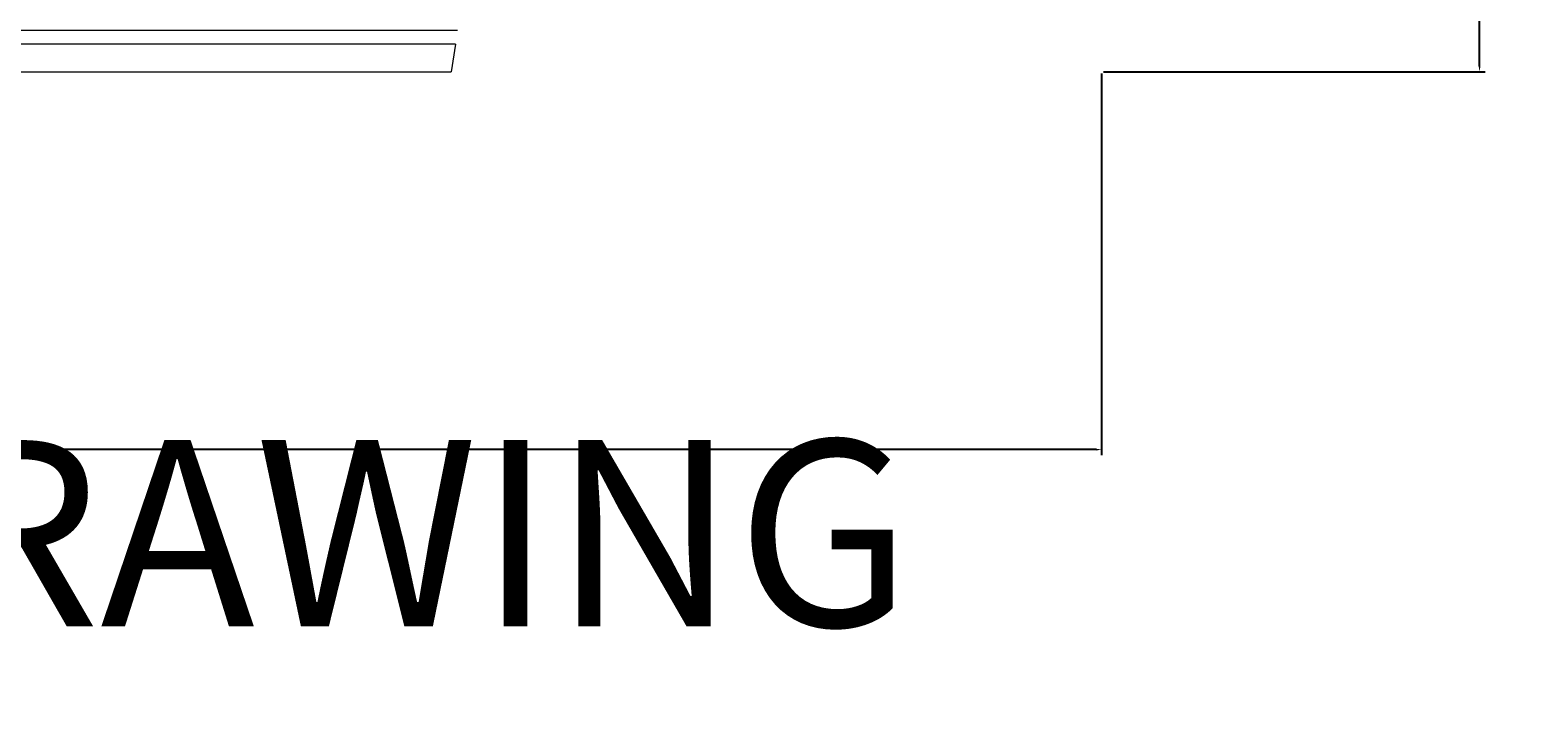
# Model space of a CAD drawing. Units: inches. Extents: x 4159 to 4826, y 299 to 1026.
# Tile 22 of 37: x 4354 to 4402, y 559 to 581. Entities that reach past the tile are written whole.
import ezdxf

# ---------------------------------------------------------------- set-up
doc = ezdxf.new("R2010")
doc.units = ezdxf.units.IN
for name, color, linetype, lineweight in [('A-ANNO-DIMS', 2, 'Continuous', 18), ('A-AREA-IDEN', 7, 'Continuous', 18), ('A-FURN', 8, 'Continuous', 18)]:
    doc.layers.add(name, color=color, linetype=linetype, lineweight=lineweight)
doc.styles.get("Standard").update_dxf_attribs({"font": 'arial.ttf'})
doc.dimstyles.get("Standard").update_dxf_attribs({"dimtxt": 0.18, "dimasz": 0.18, "dimexe": 0.18, "dimexo": 0.0625, "dimgap": 0.09, "dimtad": 0, "dimtih": 1, "dimtoh": 1, "dimdec": 4, "dimzin": 0, "dimdsep": 46, "dimtxsty": 'Standard', "dimcen": 0.09, "dimadec": 0, "dimazin": 0, "dimtfac": 1, "dimtdec": 4, "dimtofl": 0, "dimtmove": 0, "dimatfit": 3, "dimfxl": 1, "dimtolj": 1, "dimtzin": 0, "dimarcsym": 0})

# ---------------------------------------------------------------- blocks, each defined once
blk = doc.blocks.new('Dining Set - 36 x 72 in.')
for p, q in [((5.7696, -26), (22.2392, -26)), ((22.1584, -26.5), (5.8466, -26.5)), ((22.1563, -26.49967), (22, -27.5)), ((6, -27.5), (22, -27.5))]:
    blk.add_line(p, q)
blk = doc.blocks.new('*D35')
at = {"layer": 'A-ANNO-DIMS', "color": 0, "lineweight": -2, "transparency": 16777216}
for p, q in [((4307.16, 579.671), (4307.16, 567.387)), ((4388.274, 579.671), (4388.274, 567.387)), ((4307.34, 567.567), (4346.439, 567.567)), ((4388.094, 567.567), (4348.995, 567.567))]:
    blk.add_line(p, q, dxfattribs=at)
at = {"layer": 'A-ANNO-DIMS', "color": 0, "transparency": 16777216}
for points in [[(4307.34, 567.597), (4307.34, 567.537), (4307.16, 567.567)], [(4388.094, 567.597), (4388.094, 567.537), (4388.274, 567.567)]]:
    blk.add_solid(points, dxfattribs=at)
at = {"layer": 'Defpoints', "color": 0, "transparency": 16777216}
for p in [(4307.16, 579.734), (4388.274, 579.734), (4388.274, 567.567)]:
    blk.add_point(p, dxfattribs=at)
at = {"layer": 'A-ANNO-DIMS', "color": 0, "transparency": 16777216, "insert": (4347.717, 567.567), "char_height": 0.18, "attachment_point": 5}
blk.add_mtext('\\A1;DINING SET 81 TYP.', dxfattribs=at)
blk = doc.blocks.new('*D36')
at = {"layer": 'A-ANNO-DIMS', "color": 0, "lineweight": -2, "transparency": 16777216}
for p, q in [((4388.337, 628.759), (4400.621, 628.759)), ((4400.441, 628.579), (4400.441, 604.428)), ((4400.441, 579.914), (4400.441, 604.064)), ((4388.337, 579.734), (4400.621, 579.734))]:
    blk.add_line(p, q, dxfattribs=at)
at = {"layer": 'A-ANNO-DIMS', "color": 0, "transparency": 16777216}
for points in [[(4400.411, 628.579), (4400.471, 628.579), (4400.441, 628.759)], [(4400.411, 579.914), (4400.471, 579.914), (4400.441, 579.734)]]:
    blk.add_solid(points, dxfattribs=at)
at = {"layer": 'Defpoints', "color": 0, "transparency": 16777216}
for p in [(4388.274, 628.759), (4400.441, 628.759), (4388.274, 579.734)]:
    blk.add_point(p, dxfattribs=at)
at = {"layer": 'A-ANNO-DIMS', "color": 0, "transparency": 16777216, "insert": (4400.441, 604.246), "char_height": 0.18, "attachment_point": 5}
blk.add_mtext('\\A1;49 TYP.', dxfattribs=at)
blk = doc.blocks.new('*D44')
at = {"layer": 'A-ANNO-DIMS', "color": 0, "lineweight": -2, "transparency": 16777216}
for p, q in [((4287.263, 963.093), (4158.88, 963.093)), ((4159.06, 962.913), (4159.06, 647.826)), ((4159.06, 332.375), (4159.06, 647.462)), ((4447.248, 332.195), (4158.88, 332.195))]:
    blk.add_line(p, q, dxfattribs=at)
at = {"layer": 'A-ANNO-DIMS', "color": 0, "transparency": 16777216}
for points in [[(4159.03, 962.913), (4159.09, 962.913), (4159.06, 963.093)], [(4159.03, 332.375), (4159.09, 332.375), (4159.06, 332.195)]]:
    blk.add_solid(points, dxfattribs=at)
at = {"layer": 'Defpoints', "color": 0, "transparency": 16777216}
for p in [(4287.326, 963.093), (4159.06, 332.195), (4447.31, 332.195)]:
    blk.add_point(p, dxfattribs=at)
at = {"layer": 'A-ANNO-DIMS', "color": 0, "transparency": 16777216, "insert": (4159.06, 647.644), "char_height": 0.18, "attachment_point": 5}
blk.add_mtext('\\A1;630.9', dxfattribs=at)

msp = doc.modelspace()

# ---------------------------------------------------------------- block references
at = {"layer": 'A-FURN', "xscale": 0.8913588978043845, "yscale": 0.8913588978043845, "zscale": 0.8913588978043845}
msp.add_blockref('Dining Set - 36 x 72 in.', (4347.717, 604.246), dxfattribs=at)

# ---------------------------------------------------------------- texts
at = {"layer": 'A-AREA-IDEN'}
msp.add_text('DINING\\DRAWING', height=6, dxfattribs=at).set_placement((4314.093, 561.874))

# ---------------------------------------------------------------- dimensions: what is measured, and where the dimension line sits
at = {"layer": 'A-ANNO-DIMS'}
dim = msp.add_linear_dim(base=(4159.06, 332.195), p1=(4287.326, 963.093), p2=(4447.31, 332.195), angle=90, dimstyle='Standard', override={"dimdec": 1, "dimlfac": 1, "dimrnd": 0, "dimzin": 0, "dimdsep": 46, "dimlunit": 2}, dxfattribs=at)
dim.commit()
dim.dimension.update_dxf_attribs({"geometry": '*D44', "text_midpoint": (4159.06, 647.644)})
dim = msp.add_linear_dim(base=(4400.441, 628.759), p1=(4388.274, 579.734), p2=(4388.274, 628.759), angle=90, text='<> TYP.', dimstyle='Standard', override={"dimdec": 0, "dimlfac": 1, "dimrnd": 0, "dimzin": 0, "dimdsep": 46, "dimlunit": 2}, dxfattribs=at)
dim.commit()
dim.dimension.update_dxf_attribs({"geometry": '*D36', "text_midpoint": (4400.441, 604.246)})
dim = msp.add_linear_dim(base=(4388.274, 567.567), p1=(4307.16, 579.734), p2=(4388.274, 579.734), text='DINING SET <> TYP.', dimstyle='Standard', override={"dimdec": 0, "dimlfac": 1, "dimrnd": 0, "dimzin": 0, "dimdsep": 46, "dimlunit": 2}, dxfattribs=at)
dim.commit()
dim.dimension.update_dxf_attribs({"geometry": '*D35', "text_midpoint": (4347.717, 567.567)})

doc.saveas('drawing.dxf')
